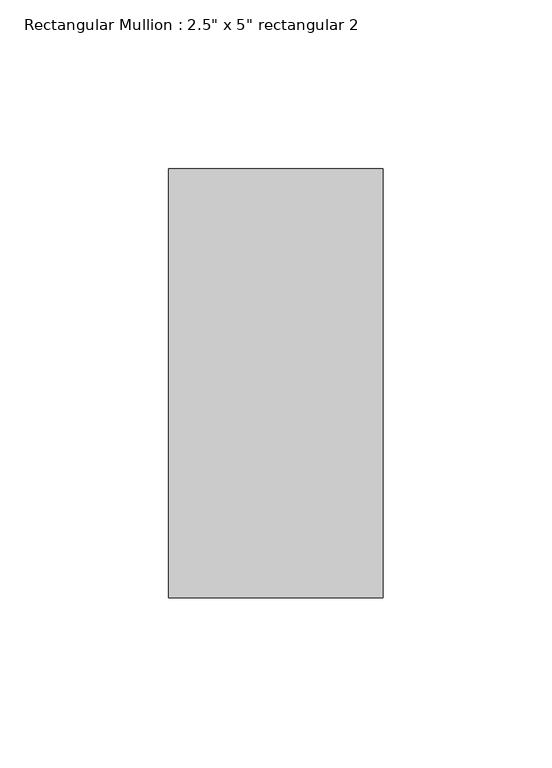
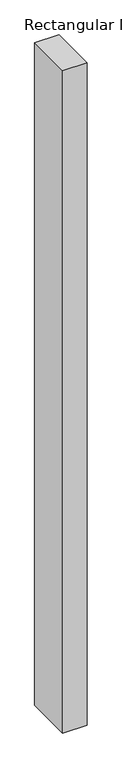
"""IFC4 building model written with IfcOpenShell, lengths in millimetres: member geometry."""

from ifc_helpers import new_model, si_unit, frame, origin, place, context, project, spatial, polyline, outline, extrude, source, transform, mapped, element, save


def member_2fae0574(model_context):
    return source(origin(), model_context, "Body", "SweptSolid", [
        extrude(outline(polyline([(0.0, 63.5), (0.0, -63.5), (-63.5, -63.5), (-63.5, 63.5), (0.0, 63.5)])), frame((0.0, 0.0, -1828.8), z_axis=(0.0, 0.0, 1.0), x_axis=(1.0, 0.0, 0.0)), (0.0, 0.0, 1.0), 1828.8),
    ])


if __name__ == "__main__":
    model = new_model("IFC4")
    model_context = context("Model", 3, world=origin())
    ifc_project = project(units=[si_unit("LENGTHUNIT", "METRE", prefix="MILLI")], contexts=[model_context])
    site = spatial("IfcSite", under=ifc_project)
    building = spatial("IfcBuilding", under=site)
    placement = place(None, origin())
    member_shape = member_2fae0574(model_context)
    element("IfcMember", 1, ObjectType="Rectangular Mullion : 2.5\" x 5\" rectangular 2", at=placement, inside=building, context=model_context, shape_type="MappedRepresentation", body=[
        mapped(member_shape, transform((0.0, 0.0, 0.0), x_axis=(1.0, 0.0, 0.0), y_axis=(0.0, 1.0, 0.0), z_axis=(0.0, 0.0, 1.0))),
    ])
    save(model, "model.ifc")

# Revit data of these elements
# Type "Rectangular Mullion : 2.5\" x 5\" rectangular 2"
#   built-in parameter 1007304 = 0.416667 (stored number, unit not read)
#   built-in parameter 1007301 = 0.104167 (stored number, unit not read)
#   built-in parameter 1007300 = 0.104167 (stored number, unit not read)
